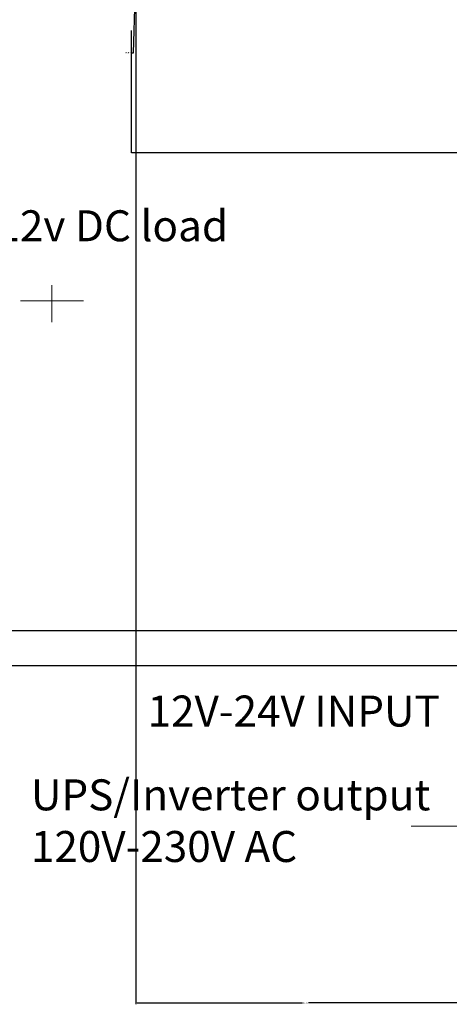
# Model space of a CAD drawing. Units: millimetres. Extents: x -8 to 285, y 5 to 221.
# Tile 16 of 30: x 130 to 186, y 5 to 132. Entities that reach past the tile are written whole.
import ezdxf

# ---------------------------------------------------------------- set-up
doc = ezdxf.new("R2010")
doc.units = ezdxf.units.MM
for name, color, linetype, lineweight in [('A-ANNO-DIMS', 2, 'Continuous', 18), ('E-ANNO-SYMB', 7, 'Continuous', 18), ('E-ANNO-TEXT', 7, 'Continuous', 18), ('E-POWR-AC-NEUT', 3, 'Continuous', 25), ('E-POWR-DC-NEG', 3, 'Continuous', 25)]:
    doc.layers.add(name, color=color, linetype=linetype, lineweight=lineweight)
doc.layers.add('E-POWR-DC-POS', color=30, linetype='Continuous', lineweight=25, true_color=0xf26722)
doc.styles.get("Standard").update_dxf_attribs({"font": 'arial.ttf'})
doc.dimstyles.get("Standard").update_dxf_attribs({"dimtxt": 0.18, "dimasz": 0.18, "dimexe": 0.18, "dimexo": 0.0625, "dimgap": 0.09, "dimtad": 0, "dimtih": 1, "dimtoh": 1, "dimdec": 4, "dimzin": 0, "dimdsep": 46, "dimtxsty": 'Standard', "dimcen": 0.09, "dimadec": 0, "dimazin": 0, "dimtfac": 1, "dimtdec": 4, "dimtofl": 0, "dimtmove": 0, "dimatfit": 3, "dimfxl": 1, "dimtolj": 1, "dimtzin": 0, "dimarcsym": 0})

# ---------------------------------------------------------------- blocks, each defined once
blk = doc.blocks.new('*D10')
at = {"layer": 'A-ANNO-DIMS', "color": 0, "lineweight": -2, "transparency": 16777216}
for p, q in [((145.1, 206.46), (-7.61, 206.46)), ((-7.43, 206.28), (-7.43, 113.16)), ((-7.43, 19.68), (-7.43, 112.8)), ((30.45, 19.5), (-7.61, 19.5))]:
    blk.add_line(p, q, dxfattribs=at)
at = {"layer": 'A-ANNO-DIMS', "color": 0, "transparency": 16777216}
for points in [[(-7.46, 206.28), (-7.4, 206.28), (-7.43, 206.46)], [(-7.46, 19.68), (-7.4, 19.68), (-7.43, 19.5)]]:
    blk.add_solid(points, dxfattribs=at)
at = {"layer": 'Defpoints', "color": 0, "transparency": 16777216}
for p in [(-7.43, 206.46), (145.17, 206.46), (30.52, 19.5)]:
    blk.add_point(p, dxfattribs=at)
at = {"layer": 'A-ANNO-DIMS', "color": 0, "transparency": 16777216, "insert": (-7.43, 112.98), "char_height": 0.18, "attachment_point": 5}
blk.add_mtext('\\A1;186.95', dxfattribs=at)
blk = doc.blocks.new('*D13')
at = {"layer": 'A-ANNO-DIMS', "color": 0, "lineweight": -2, "transparency": 16777216}
for p, q in [((145.21, 137.01), (145.21, 5.22)), ((189.04, 137.01), (189.04, 5.22)), ((145.39, 5.4), (166.73, 5.4)), ((188.86, 5.4), (167.52, 5.4))]:
    blk.add_line(p, q, dxfattribs=at)
at = {"layer": 'A-ANNO-DIMS', "color": 0, "transparency": 16777216}
for points in [[(145.39, 5.43), (145.39, 5.37), (145.21, 5.4)], [(188.86, 5.43), (188.86, 5.37), (189.04, 5.4)]]:
    blk.add_solid(points, dxfattribs=at)
at = {"layer": 'Defpoints', "color": 0, "transparency": 16777216}
for p in [(145.21, 137.08), (189.04, 137.08), (189.04, 5.4)]:
    blk.add_point(p, dxfattribs=at)
at = {"layer": 'A-ANNO-DIMS', "color": 0, "transparency": 16777216, "insert": (167.12, 5.4), "char_height": 0.18, "attachment_point": 5}
blk.add_mtext('\\A1;43.83', dxfattribs=at)
blk = doc.blocks.new('*D29')
at = {"layer": 'A-ANNO-DIMS', "color": 0, "lineweight": -2, "transparency": 16777216}
for p, q in [((145.6, 152.07), (145.78, 152.07)), ((145.69, 151.98), (145.69, 152.16)), ((144.92, 128.08), (145.2, 136.9)), ((144.74, 128.08), (144.92, 128.08))]:
    blk.add_line(p, q, dxfattribs=at)
at = {"layer": 'A-ANNO-DIMS', "color": 0, "transparency": 16777216}
blk.add_solid([(145.17, 136.9), (145.23, 136.89), (145.21, 137.08)], dxfattribs=at)
at = {"layer": 'Defpoints', "color": 0, "transparency": 16777216}
for p in [(145.69, 152.07), (145.21, 137.08)]:
    blk.add_point(p, dxfattribs=at)
at = {"layer": 'A-ANNO-DIMS', "color": 0, "transparency": 16777216, "insert": (144.24, 128.08), "char_height": 0.18, "attachment_point": 5}
blk.add_mtext('\\A1;6X R15', dxfattribs=at)

msp = doc.modelspace()

# ---------------------------------------------------------------- linework, layer by layer
at = {"layer": 'E-ANNO-SYMB'}
for p, q in [((134.392, 93.2998), (134.392, 98.0907)), ((130.3321, 96.0531), (138.4519, 96.0531)), ((134.392, 96.0531), (134.392, 93.2998))]:
    msp.add_line(p, q, dxfattribs=at)
at = {"layer": 'E-ANNO-TEXT'}
msp.add_lwpolyline([(237.8513, 44.4759), (237.8513, 28.2311), (180.7415, 28.2311)], dxfattribs=at)
at = {"layer": 'E-POWR-AC-NEUT'}
msp.add_lwpolyline([(231.5468, 34.6512), (231.5468, 58.5666), (262.873, 58.5666), (262.873, 115.1427), (144.6762, 115.1427), (144.6762, 130.9614)], dxfattribs=at)
at = {"layer": 'E-POWR-DC-NEG'}
msp.add_line((58.1717, 53.4644), (215.8749, 53.4644), dxfattribs=at)
at = {"layer": 'E-POWR-DC-POS'}
msp.add_lwpolyline([(52.1717, 48.962), (202.4345, 48.962), (202.4345, 34.9746)], dxfattribs=at)

# ---------------------------------------------------------------- texts
at = {"layer": 'E-ANNO-TEXT', "char_height": 4, "attachment_point": 1}
for s, width, insert in [('DC output 12v DC load', 65.111825, (100.1263, 107.7354)), ('12V-24V INPUT', 39.615541, (146.7437, 45.0874)), ('UPS/Inverter output \\P120V-230V AC ', 54.163791, (131.6826, 34.2645))]:
    msp.add_mtext_dynamic_manual_height_columns(s, width=width, gutter_width=12.5, heights=[0], dxfattribs=dict(at, insert=insert))

# ---------------------------------------------------------------- dimensions: what is measured, and where the dimension line sits
at = {"layer": 'A-ANNO-DIMS'}
dim = msp.add_linear_dim(base=(-7.4275, 206.4568), p1=(30.516, 19.502), p2=(145.1651, 206.4568), angle=90, dimstyle='Standard', override={"dimdec": 2, "dimlfac": 1, "dimrnd": 0, "dimzin": 0, "dimdsep": 46, "dimlunit": 2}, dxfattribs=at)
dim.commit()
dim.dimension.update_dxf_attribs({"geometry": '*D10', "text_midpoint": (-7.4275, 112.9794)})
dim = msp.add_radius_dim(center=(145.6897, 152.0675), mpoint=(145.21, 137.0752), text='6X <>', dimstyle='Standard', override={"dimdec": 0, "dimlfac": 1, "dimrnd": 0, "dimzin": 0, "dimdsep": 46, "dimlunit": 2}, dxfattribs=at)
dim.commit()
dim.dimension.update_dxf_attribs({"geometry": '*D29', "text_midpoint": (144.2426, 128.0798), "dimtype": 164})
dim = msp.add_linear_dim(base=(189.039, 5.402), p1=(145.2095, 137.0752), p2=(189.039, 137.0752), dimstyle='Standard', override={"dimdec": 2, "dimlfac": 1, "dimrnd": 0, "dimzin": 0, "dimdsep": 46, "dimlunit": 2}, dxfattribs=at)
dim.commit()
dim.dimension.update_dxf_attribs({"geometry": '*D13', "text_midpoint": (167.1243, 5.402)})

doc.saveas('drawing.dxf')
